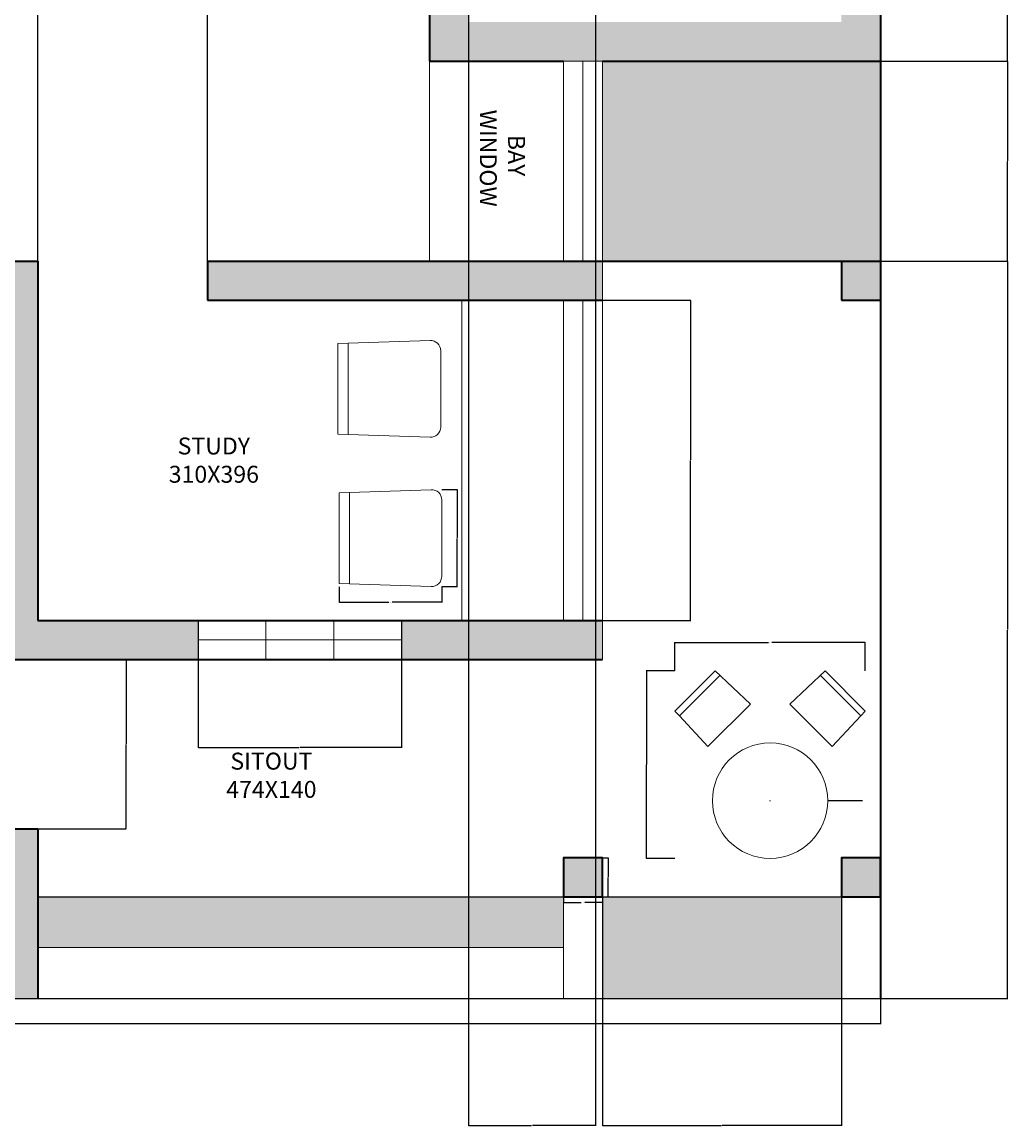
# Model space of a CAD drawing. Units: centimetres. Extents: x 2178 to 3635, y 1064 to 2635.
# Tile 4 of 9: x 3053 to 3635, y 1113 to 1765. Entities that reach past the tile are written whole.
import ezdxf

# ---------------------------------------------------------------- set-up
doc = ezdxf.new("R2010")
doc.units = ezdxf.units.CM
for name, color, linetype, lineweight in [('A-ANNO-DIMS', 2, 'Continuous', 18), ('A-ANNO-TEXT', 7, 'Continuous', 18), ('A-AREA-IDEN', 7, 'Continuous', 18), ('A-COLS', 7, 'Continuous', 35), ('A-FLOR', 7, 'Continuous', 25), ('A-FLOR-CASE', 32, 'Continuous', 18), ('A-FLOR-PATT', 95, 'Continuous', 13), ('A-FLOR-STRS', 7, 'Continuous', 18), ('A-FURN', 42, 'Continuous', 18), ('A-GLAZ', 4, 'Continuous', 18), ('A-WALL', 7, 'Continuous', 35)]:
    doc.layers.add(name, color=color, linetype=linetype, lineweight=lineweight)
doc.layers.add('A-WALL-PATT', color=18, linetype='Continuous', lineweight=13, true_color=0x000000)
doc.styles.get("Standard").update_dxf_attribs({"font": 'arial.ttf'})
doc.dimstyles.get("Standard").update_dxf_attribs({"dimtxt": 0.18, "dimasz": 0.18, "dimexe": 0.18, "dimexo": 0.0625, "dimgap": 0.09, "dimtad": 0, "dimtih": 1, "dimtoh": 1, "dimdec": 4, "dimzin": 0, "dimdsep": 46, "dimtxsty": 'Standard', "dimcen": 0.09, "dimadec": 0, "dimazin": 0, "dimtfac": 1, "dimtdec": 4, "dimtofl": 0, "dimtmove": 0, "dimatfit": 3, "dimfxl": 1, "dimtolj": 1, "dimtzin": 0, "dimarcsym": 0})

# ---------------------------------------------------------------- blocks, each defined once
blk = doc.blocks.new('chair')
for p, q in [((3410.95, 1354.53), (3434.84, 1378.41)), ((3434.84, 1378.41), (3410.95, 1354.53)), ((3494.17, 1378.41), (3518.06, 1354.53)), ((3518.06, 1354.53), (3494.17, 1378.41))]:
    blk.add_line(p, q)
for points in [[(3432.06, 1381.01), (3452.88, 1361.54), (3427.83, 1336.49), (3410.95, 1354.53), (3408.36, 1357.3)], [(3496.95, 1381.01), (3476.13, 1361.54), (3501.18, 1336.49), (3518.06, 1354.53), (3520.65, 1357.3)]]:
    blk.add_lwpolyline(points, close=True)
blk.add_circle((3464.51, 1304.51), 34.04)
blk = doc.blocks.new('c')
blk.add_lwpolyline([(3808.85, 1833.77), (3776.18, 1834.86), (3776.18, 1867.04), (3808.85, 1868.12, -0.424007), (3812.61, 1864.48), (3812.61, 1837.41, -0.424007)], format="xyb", close=True)
blk.add_lwpolyline([(3779.83, 1867.16), (3779.83, 1834.74)])
blk = doc.blocks.new('COL-0230-SQ')
blk.add_lwpolyline([(0, 0), (23, 0), (23, 23), (0, 23)], close=True)
blk = doc.blocks.new('*D20')
at = {"layer": 'A-ANNO-DIMS', "color": 0, "lineweight": -2, "transparency": 16777216}
for p, q in [((3240.31, 1431.49), (3240.31, 1422.28)), ((3300.89, 1431.49), (3300.89, 1422.28)), ((3240.49, 1422.46), (3269.64, 1422.46)), ((3300.71, 1422.46), (3271.55, 1422.46))]:
    blk.add_line(p, q, dxfattribs=at)
at = {"layer": 'A-ANNO-DIMS', "color": 0, "transparency": 16777216}
for points in [[(3240.49, 1422.49), (3240.49, 1422.43), (3240.31, 1422.46)], [(3300.71, 1422.49), (3300.71, 1422.43), (3300.89, 1422.46)]]:
    blk.add_solid(points, dxfattribs=at)
at = {"layer": 'Defpoints', "color": 0, "transparency": 16777216}
for p in [(3240.31, 1431.55), (3300.89, 1431.55), (3300.89, 1422.46)]:
    blk.add_point(p, dxfattribs=at)
at = {"layer": 'A-ANNO-DIMS', "color": 0, "transparency": 16777216, "insert": (3270.6, 1422.46), "char_height": 0.18, "attachment_point": 5}
blk.add_mtext('\\A1;CHAIR 61 TYP.', dxfattribs=at)
blk = doc.blocks.new('*D21')
at = {"layer": 'A-ANNO-DIMS', "color": 0, "lineweight": -2, "transparency": 16777216}
for p, q in [((3300.95, 1488.8), (3310.16, 1488.8)), ((3309.98, 1488.62), (3309.98, 1460.36)), ((3309.98, 1431.73), (3309.98, 1459.99)), ((3300.95, 1431.55), (3310.16, 1431.55))]:
    blk.add_line(p, q, dxfattribs=at)
at = {"layer": 'A-ANNO-DIMS', "color": 0, "transparency": 16777216}
for points in [[(3309.95, 1488.62), (3310.01, 1488.62), (3309.98, 1488.8)], [(3309.95, 1431.73), (3310.01, 1431.73), (3309.98, 1431.55)]]:
    blk.add_solid(points, dxfattribs=at)
at = {"layer": 'Defpoints', "color": 0, "transparency": 16777216}
for p in [(3300.89, 1488.8), (3309.98, 1488.8), (3300.89, 1431.55)]:
    blk.add_point(p, dxfattribs=at)
at = {"layer": 'A-ANNO-DIMS', "color": 0, "transparency": 16777216, "insert": (3309.98, 1460.17), "char_height": 0.18, "attachment_point": 5}
blk.add_mtext('\\A1;57 TYP.', dxfattribs=at)
blk = doc.blocks.new('*D38')
at = {"layer": 'A-ANNO-DIMS', "color": 0, "lineweight": -2, "transparency": 16777216}
for p, q in [((3372.6, 1248.53), (3372.6, 1244.96)), ((3372.78, 1245.14), (3383, 1245.14)), ((3395.42, 1245.14), (3385.21, 1245.14)), ((3395.6, 1248.53), (3395.6, 1244.96))]:
    blk.add_line(p, q, dxfattribs=at)
at = {"layer": 'A-ANNO-DIMS', "color": 0, "transparency": 16777216}
for points in [[(3372.78, 1245.17), (3372.78, 1245.11), (3372.6, 1245.14)], [(3395.42, 1245.17), (3395.42, 1245.11), (3395.6, 1245.14)]]:
    blk.add_solid(points, dxfattribs=at)
at = {"layer": 'Defpoints', "color": 0, "transparency": 16777216}
for p in [(3372.6, 1248.59), (3395.6, 1248.59), (3395.6, 1245.14)]:
    blk.add_point(p, dxfattribs=at)
at = {"layer": 'A-ANNO-DIMS', "color": 0, "transparency": 16777216, "insert": (3384.1, 1245.14), "char_height": 0.18, "attachment_point": 5}
blk.add_mtext('\\A1;COLUMN 23 TYP.', dxfattribs=at)
blk = doc.blocks.new('*D39')
at = {"layer": 'A-ANNO-DIMS', "color": 0, "lineweight": -2, "transparency": 16777216}
for p, q in [((3395.67, 1271.59), (3399.23, 1271.59)), ((3399.05, 1271.41), (3399.05, 1260.27)), ((3399.05, 1248.77), (3399.05, 1259.91)), ((3395.67, 1248.59), (3399.23, 1248.59))]:
    blk.add_line(p, q, dxfattribs=at)
at = {"layer": 'A-ANNO-DIMS', "color": 0, "transparency": 16777216}
for points in [[(3399.02, 1271.41), (3399.08, 1271.41), (3399.05, 1271.59)], [(3399.02, 1248.77), (3399.08, 1248.77), (3399.05, 1248.59)]]:
    blk.add_solid(points, dxfattribs=at)
at = {"layer": 'Defpoints', "color": 0, "transparency": 16777216}
for p in [(3395.6, 1271.59), (3399.05, 1271.59), (3395.6, 1248.59)]:
    blk.add_point(p, dxfattribs=at)
at = {"layer": 'A-ANNO-DIMS', "color": 0, "transparency": 16777216, "insert": (3399.05, 1260.09), "char_height": 0.18, "attachment_point": 5}
blk.add_mtext('\\A1;23 TYP.', dxfattribs=at)
blk = doc.blocks.new('*D42')
at = {"layer": 'A-ANNO-DIMS', "color": 0, "lineweight": -2, "transparency": 16777216}
for p, q in [((3438.42, 1381.84), (3438.42, 1398.8)), ((3438.6, 1398.62), (3493.59, 1398.62)), ((3550.53, 1398.62), (3495.54, 1398.62)), ((3550.71, 1381.84), (3550.71, 1398.8))]:
    blk.add_line(p, q, dxfattribs=at)
at = {"layer": 'A-ANNO-DIMS', "color": 0, "transparency": 16777216}
for points in [[(3438.6, 1398.65), (3438.6, 1398.59), (3438.42, 1398.62)], [(3550.53, 1398.65), (3550.53, 1398.59), (3550.71, 1398.62)]]:
    blk.add_solid(points, dxfattribs=at)
at = {"layer": 'Defpoints', "color": 0, "transparency": 16777216}
for p in [(3550.71, 1398.62), (3438.42, 1381.78), (3550.71, 1381.78)]:
    blk.add_point(p, dxfattribs=at)
at = {"layer": 'A-ANNO-DIMS', "color": 0, "transparency": 16777216, "insert": (3494.56, 1398.62), "char_height": 0.18, "attachment_point": 5}
blk.add_mtext('\\A1;PATIO SET 112', dxfattribs=at)
blk = doc.blocks.new('*D43')
at = {"layer": 'A-ANNO-DIMS', "color": 0, "lineweight": -2, "transparency": 16777216}
for p, q in [((3438.35, 1381.78), (3421.39, 1381.78)), ((3421.57, 1381.6), (3421.57, 1326.69)), ((3421.57, 1271.43), (3421.57, 1326.33)), ((3438.35, 1271.25), (3421.39, 1271.25))]:
    blk.add_line(p, q, dxfattribs=at)
at = {"layer": 'A-ANNO-DIMS', "color": 0, "transparency": 16777216}
for points in [[(3421.54, 1381.6), (3421.6, 1381.6), (3421.57, 1381.78)], [(3421.54, 1271.43), (3421.6, 1271.43), (3421.57, 1271.25)]]:
    blk.add_solid(points, dxfattribs=at)
at = {"layer": 'Defpoints', "color": 0, "transparency": 16777216}
for p in [(3421.57, 1381.78), (3438.42, 1381.78), (3438.42, 1271.25)]:
    blk.add_point(p, dxfattribs=at)
at = {"layer": 'A-ANNO-DIMS', "color": 0, "transparency": 16777216, "insert": (3421.57, 1326.51), "char_height": 0.18, "attachment_point": 5}
blk.add_mtext('\\A1;111', dxfattribs=at)
blk = doc.blocks.new('*D46')
at = {"layer": 'A-ANNO-DIMS', "color": 0, "lineweight": -2, "transparency": 16777216}
for p, q in [((2253.6, 1248.53), (2253.6, 1173.41)), ((3559.6, 1248.53), (3559.6, 1173.41)), ((2253.78, 1173.59), (2906.25, 1173.59)), ((3559.42, 1173.59), (2906.95, 1173.59))]:
    blk.add_line(p, q, dxfattribs=at)
at = {"layer": 'A-ANNO-DIMS', "color": 0, "transparency": 16777216}
for points in [[(2253.78, 1173.62), (2253.78, 1173.56), (2253.6, 1173.59)], [(3559.42, 1173.62), (3559.42, 1173.56), (3559.6, 1173.59)]]:
    blk.add_solid(points, dxfattribs=at)
at = {"layer": 'Defpoints', "color": 0, "transparency": 16777216}
for p in [(2253.6, 1248.59), (3559.6, 1248.59), (2253.6, 1173.59)]:
    blk.add_point(p, dxfattribs=at)
at = {"layer": 'A-ANNO-DIMS', "color": 0, "transparency": 16777216, "insert": (2906.6, 1173.59), "char_height": 0.18, "attachment_point": 5}
blk.add_mtext('\\A1;1306', dxfattribs=at)
blk = doc.blocks.new('*D58')
at = {"layer": 'A-ANNO-DIMS', "color": 0, "lineweight": -2, "transparency": 16777216}
for p, q in [((3559.67, 1797.09), (3634.78, 1797.09)), ((3634.6, 1796.91), (3634.6, 1769.52)), ((3634.6, 1741.77), (3634.6, 1769.16)), ((3559.67, 1741.59), (3634.78, 1741.59))]:
    blk.add_line(p, q, dxfattribs=at)
at = {"layer": 'A-ANNO-DIMS', "color": 0, "transparency": 16777216}
for points in [[(3634.57, 1796.91), (3634.63, 1796.91), (3634.6, 1797.09)], [(3634.57, 1741.77), (3634.63, 1741.77), (3634.6, 1741.59)]]:
    blk.add_solid(points, dxfattribs=at)
at = {"layer": 'Defpoints', "color": 0, "transparency": 16777216}
for p in [(3559.6, 1797.09), (3634.6, 1797.09), (3559.6, 1741.59)]:
    blk.add_point(p, dxfattribs=at)
at = {"layer": 'A-ANNO-DIMS', "color": 0, "transparency": 16777216, "insert": (3634.6, 1769.34), "char_height": 0.18, "attachment_point": 5}
blk.add_mtext('\\A1;55.5', dxfattribs=at)
blk = doc.blocks.new('*D59')
at = {"layer": 'A-ANNO-DIMS', "color": 0, "lineweight": -2, "transparency": 16777216}
for p, q in [((3559.67, 1741.59), (3634.78, 1741.59)), ((3634.6, 1741.41), (3634.6, 1682.77)), ((3634.6, 1623.77), (3634.6, 1682.41)), ((3559.67, 1623.59), (3634.78, 1623.59))]:
    blk.add_line(p, q, dxfattribs=at)
at = {"layer": 'A-ANNO-DIMS', "color": 0, "transparency": 16777216}
for points in [[(3634.57, 1741.41), (3634.63, 1741.41), (3634.6, 1741.59)], [(3634.57, 1623.77), (3634.63, 1623.77), (3634.6, 1623.59)]]:
    blk.add_solid(points, dxfattribs=at)
at = {"layer": 'Defpoints', "color": 0, "transparency": 16777216}
for p in [(3559.6, 1741.59), (3634.6, 1741.59), (3559.6, 1623.59)]:
    blk.add_point(p, dxfattribs=at)
at = {"layer": 'A-ANNO-DIMS', "color": 0, "transparency": 16777216, "insert": (3634.6, 1682.59), "char_height": 0.18, "attachment_point": 5}
blk.add_mtext('\\A1;118', dxfattribs=at)
blk = doc.blocks.new('*D60')
at = {"layer": 'A-ANNO-DIMS', "color": 0, "lineweight": -2, "transparency": 16777216}
for p, q in [((3559.67, 1623.59), (3634.78, 1623.59)), ((3634.6, 1623.41), (3634.6, 1406.27)), ((3634.6, 1188.77), (3634.6, 1405.91)), ((3559.67, 1188.59), (3634.78, 1188.59))]:
    blk.add_line(p, q, dxfattribs=at)
at = {"layer": 'A-ANNO-DIMS', "color": 0, "transparency": 16777216}
for points in [[(3634.57, 1623.41), (3634.63, 1623.41), (3634.6, 1623.59)], [(3634.57, 1188.77), (3634.63, 1188.77), (3634.6, 1188.59)]]:
    blk.add_solid(points, dxfattribs=at)
at = {"layer": 'Defpoints', "color": 0, "transparency": 16777216}
for p in [(3559.6, 1623.59), (3634.6, 1623.59), (3559.6, 1188.59)]:
    blk.add_point(p, dxfattribs=at)
at = {"layer": 'A-ANNO-DIMS', "color": 0, "transparency": 16777216, "insert": (3634.6, 1406.09), "char_height": 0.18, "attachment_point": 5}
blk.add_mtext('\\A1;435', dxfattribs=at)
blk = doc.blocks.new('*D62')
at = {"layer": 'A-ANNO-DIMS', "color": 0, "lineweight": -2, "transparency": 16777216}
for p, q in [((3062.6, 1623.65), (3062.6, 2634.77)), ((3062.78, 2634.59), (3112.32, 2634.59)), ((3162.42, 2634.59), (3112.88, 2634.59)), ((3162.6, 1623.65), (3162.6, 2634.77))]:
    blk.add_line(p, q, dxfattribs=at)
at = {"layer": 'A-ANNO-DIMS', "color": 0, "transparency": 16777216}
for points in [[(3062.78, 2634.62), (3062.78, 2634.56), (3062.6, 2634.59)], [(3162.42, 2634.62), (3162.42, 2634.56), (3162.6, 2634.59)]]:
    blk.add_solid(points, dxfattribs=at)
at = {"layer": 'Defpoints', "color": 0, "transparency": 16777216}
for p in [(3162.6, 2634.59), (3062.6, 1623.59), (3162.6, 1623.59)]:
    blk.add_point(p, dxfattribs=at)
at = {"layer": 'A-ANNO-DIMS', "color": 0, "transparency": 16777216, "insert": (3112.6, 2634.59), "char_height": 0.18, "attachment_point": 5}
blk.add_mtext('\\A1;100', dxfattribs=at)
blk = doc.blocks.new('*D67')
at = {"layer": 'A-ANNO-DIMS', "color": 0, "lineweight": -2, "transparency": 16777216}
for p, q in [((3316.6, 1927.53), (3316.6, 1113.41)), ((3391.6, 1927.53), (3391.6, 1113.41)), ((3316.78, 1113.59), (3353.89, 1113.59)), ((3391.42, 1113.59), (3354.32, 1113.59))]:
    blk.add_line(p, q, dxfattribs=at)
at = {"layer": 'A-ANNO-DIMS', "color": 0, "transparency": 16777216}
for points in [[(3316.78, 1113.62), (3316.78, 1113.56), (3316.6, 1113.59)], [(3391.42, 1113.62), (3391.42, 1113.56), (3391.6, 1113.59)]]:
    blk.add_solid(points, dxfattribs=at)
at = {"layer": 'Defpoints', "color": 0, "transparency": 16777216}
for p in [(3316.6, 1927.59), (3391.6, 1927.59), (3391.6, 1113.59)]:
    blk.add_point(p, dxfattribs=at)
at = {"layer": 'A-ANNO-DIMS', "color": 0, "transparency": 16777216, "insert": (3354.1, 1113.59), "char_height": 0.18, "attachment_point": 5}
blk.add_mtext('\\A1;75', dxfattribs=at)
blk = doc.blocks.new('*D68')
at = {"layer": 'A-ANNO-DIMS', "color": 0, "lineweight": -2, "transparency": 16777216}
for p, q in [((3372.67, 1600.59), (3447.78, 1600.59)), ((3447.6, 1600.41), (3447.6, 1506.27)), ((3447.6, 1411.77), (3447.6, 1505.91)), ((3372.67, 1411.59), (3447.78, 1411.59))]:
    blk.add_line(p, q, dxfattribs=at)
at = {"layer": 'A-ANNO-DIMS', "color": 0, "transparency": 16777216}
for points in [[(3447.57, 1600.41), (3447.63, 1600.41), (3447.6, 1600.59)], [(3447.57, 1411.77), (3447.63, 1411.77), (3447.6, 1411.59)]]:
    blk.add_solid(points, dxfattribs=at)
at = {"layer": 'Defpoints', "color": 0, "transparency": 16777216}
for p in [(3372.6, 1600.59), (3372.6, 1411.59), (3447.6, 1411.59)]:
    blk.add_point(p, dxfattribs=at)
at = {"layer": 'A-ANNO-DIMS', "color": 0, "transparency": 16777216, "insert": (3447.6, 1506.09), "char_height": 0.18, "attachment_point": 5}
blk.add_mtext('\\A1;189', dxfattribs=at)
blk = doc.blocks.new('*D78')
at = {"layer": 'A-ANNO-DIMS', "color": 0, "lineweight": -2, "transparency": 16777216}
for p, q in [((3039.67, 1388.59), (3114.78, 1388.59)), ((3114.6, 1388.41), (3114.6, 1338.77)), ((3114.6, 1288.77), (3114.6, 1338.41)), ((3039.67, 1288.59), (3114.78, 1288.59))]:
    blk.add_line(p, q, dxfattribs=at)
at = {"layer": 'A-ANNO-DIMS', "color": 0, "transparency": 16777216}
for points in [[(3114.57, 1388.41), (3114.63, 1388.41), (3114.6, 1388.59)], [(3114.57, 1288.77), (3114.63, 1288.77), (3114.6, 1288.59)]]:
    blk.add_solid(points, dxfattribs=at)
at = {"layer": 'Defpoints', "color": 0, "transparency": 16777216}
for p in [(3039.6, 1388.59), (3039.6, 1288.59), (3114.6, 1288.59)]:
    blk.add_point(p, dxfattribs=at)
at = {"layer": 'A-ANNO-DIMS', "color": 0, "transparency": 16777216, "insert": (3114.6, 1338.59), "char_height": 0.18, "attachment_point": 5}
blk.add_mtext('\\A1;100', dxfattribs=at)
blk = doc.blocks.new('*D79')
at = {"layer": 'A-ANNO-DIMS', "color": 0, "lineweight": -2, "transparency": 16777216}
for p, q in [((3395.6, 1248.53), (3395.6, 1113.41)), ((3536.6, 1248.53), (3536.6, 1113.41)), ((3395.78, 1113.59), (3465.84, 1113.59)), ((3536.42, 1113.59), (3466.37, 1113.59))]:
    blk.add_line(p, q, dxfattribs=at)
at = {"layer": 'A-ANNO-DIMS', "color": 0, "transparency": 16777216}
for points in [[(3395.78, 1113.62), (3395.78, 1113.56), (3395.6, 1113.59)], [(3536.42, 1113.62), (3536.42, 1113.56), (3536.6, 1113.59)]]:
    blk.add_solid(points, dxfattribs=at)
at = {"layer": 'Defpoints', "color": 0, "transparency": 16777216}
for p in [(3395.6, 1248.59), (3536.6, 1248.59), (3536.6, 1113.59)]:
    blk.add_point(p, dxfattribs=at)
at = {"layer": 'A-ANNO-DIMS', "color": 0, "transparency": 16777216, "insert": (3466.1, 1113.59), "char_height": 0.18, "attachment_point": 5}
blk.add_mtext('\\A1;141', dxfattribs=at)
blk = doc.blocks.new('*D80')
at = {"layer": 'A-ANNO-DIMS', "color": 0, "lineweight": -2, "transparency": 16777216}
for p, q in [((3157.1, 1411.53), (3157.1, 1336.41)), ((3277.1, 1411.53), (3277.1, 1336.41)), ((3157.28, 1336.59), (3216.82, 1336.59)), ((3276.92, 1336.59), (3217.38, 1336.59))]:
    blk.add_line(p, q, dxfattribs=at)
at = {"layer": 'A-ANNO-DIMS', "color": 0, "transparency": 16777216}
for points in [[(3157.28, 1336.62), (3157.28, 1336.56), (3157.1, 1336.59)], [(3276.92, 1336.62), (3276.92, 1336.56), (3277.1, 1336.59)]]:
    blk.add_solid(points, dxfattribs=at)
at = {"layer": 'Defpoints', "color": 0, "transparency": 16777216}
for p in [(3157.1, 1411.59), (3277.1, 1411.59), (3157.1, 1336.59)]:
    blk.add_point(p, dxfattribs=at)
at = {"layer": 'A-ANNO-DIMS', "color": 0, "transparency": 16777216, "insert": (3217.1, 1336.59), "char_height": 0.18, "attachment_point": 5}
blk.add_mtext('\\A1;120', dxfattribs=at)
blk = doc.blocks.new('*D85')
at = {"layer": 'A-ANNO-DIMS', "color": 0, "lineweight": -2, "transparency": 16777216}
for p, q in [((3494.47, 1305.28), (3494.65, 1305.28)), ((3494.56, 1305.19), (3494.56, 1305.37)), ((3549.02, 1305.28), (3528.78, 1305.28))]:
    blk.add_line(p, q, dxfattribs=at)
at = {"layer": 'A-ANNO-DIMS', "color": 0, "transparency": 16777216}
blk.add_solid([(3528.78, 1305.31), (3528.78, 1305.25), (3528.6, 1305.28)], dxfattribs=at)
at = {"layer": 'Defpoints', "color": 0, "transparency": 16777216}
for p in [(3460.53, 1305.28), (3528.6, 1305.28)]:
    blk.add_point(p, dxfattribs=at)
at = {"layer": 'A-ANNO-DIMS', "color": 0, "transparency": 16777216, "insert": (3549.51, 1305.28), "char_height": 0.18, "attachment_point": 5}
blk.add_mtext('\\A1;∅68.07', dxfattribs=at)

msp = doc.modelspace()

# ---------------------------------------------------------------- hatches: boundary and pattern name
at = {"layer": 'A-FLOR-PATT'}
h = msp.add_hatch(color=256, dxfattribs=at)
h.dxf.hatch_style = 1
h.paths.add_polyline_path([(3559.605, 1741.59), (3395.605, 1741.59), (3395.605, 1623.59), (3559.605, 1623.59)])
h.paths.add_polyline_path([(3536.605, 1248.59), (3395.605, 1248.59), (3395.605, 1188.59), (3536.605, 1188.59)])
h.paths.add_polyline_path([(2636.605, 1248.59), (2253.605, 1248.59), (2253.605, 1188.59), (2636.605, 1188.59)])
at = {"layer": 'A-WALL-PATT'}
h = msp.add_hatch(color=256, dxfattribs=at)
h.dxf.hatch_style = 1
h.paths.add_polyline_path([(2276.605, 2499.59), (2253.605, 2499.59), (2253.605, 2476.59), (2276.605, 2476.59)])
h.paths.add_polyline_path([(2411.605, 2350.59), (2253.605, 2350.59), (2253.605, 2327.59), (2411.605, 2327.59)])
h.paths.add_polyline_path([(2276.605, 2252.59), (2253.605, 2252.59), (2253.605, 2020.59), (2276.605, 2020.59), (2276.605, 2093.59), (2561.605, 2093.59), (2561.605, 2116.59), (2276.605, 2116.59)])
h.paths.add_polyline_path([(2659.605, 1787.59), (2610.616, 1787.59), (2276.605, 1787.59), (2276.605, 1860.59), (2253.605, 1860.59), (2253.605, 1732.09), (2276.605, 1732.09), (2276.605, 1764.59), (2516.605, 1764.59), (2516.605, 1699.59), (2539.605, 1699.59), (2539.605, 1764.59), (2659.605, 1764.59)])
h.paths.add_polyline_path([(2539.605, 1624.59), (2276.605, 1624.59), (2276.605, 1657.09), (2253.605, 1657.09), (2253.605, 1561.59), (2276.605, 1561.59), (2276.605, 1601.59), (2539.605, 1601.59)])
h.paths.add_polyline_path([(2276.605, 1501.59), (2253.605, 1501.59), (2253.605, 1371.59), (2276.605, 1371.59)])
h.paths.add_polyline_path([(2376.605, 1271.59), (2276.605, 1271.59), (2276.605, 1311.59), (2253.605, 1311.59), (2253.605, 1248.59), (2376.605, 1248.59)])
h.paths.add_polyline_path([(2636.605, 1271.59), (2536.605, 1271.59), (2536.605, 1248.59), (2636.605, 1248.59)])
h.paths.add_polyline_path([(2659.605, 1600.59), (2919.605, 1600.59), (2919.605, 1623.59), (2636.605, 1623.59), (2636.605, 1188.59), (2659.605, 1188.59)])
h.paths.add_polyline_path([(2939.605, 1211.59), (2759.605, 1211.59), (2759.605, 1188.59), (2939.605, 1188.59)])
h.paths.add_polyline_path([(3062.605, 1288.59), (3039.605, 1288.59), (3039.605, 1188.59), (3062.605, 1188.59)])
h.paths.add_polyline_path([(3372.605, 1248.59), (3062.605, 1248.59), (3062.605, 1218.59), (3372.605, 1218.59)])
h.paths.add_polyline_path([(3395.605, 1271.59), (3372.605, 1271.59), (3372.605, 1248.59), (3395.605, 1248.59)])
h.paths.add_polyline_path([(3559.605, 1271.59), (3536.605, 1271.59), (3536.605, 1248.59), (3559.605, 1248.59)])
h.paths.add_polyline_path([(3559.605, 1623.59), (3536.605, 1623.59), (3536.605, 1600.59), (3559.605, 1600.59)])
h.paths.add_polyline_path([(3395.605, 1623.59), (3162.605, 1623.59), (3162.605, 1600.59), (3395.605, 1600.59)])
h.paths.add_polyline_path([(3395.605, 1411.59), (3277.1, 1411.59), (3277.1, 1388.59), (3395.605, 1388.59)])
h.paths.add_polyline_path([(3157.1, 1411.59), (3062.605, 1411.59), (3062.605, 1623.59), (3039.605, 1623.59), (3039.605, 1388.59), (3157.1, 1388.59)])
h.paths.add_polyline_path([(3559.605, 1797.09), (3536.605, 1797.09), (3536.605, 1764.59), (3316.605, 1764.59), (3316.605, 1927.59), (3293.605, 1927.59), (3293.605, 1741.59), (3372.605, 1741.59), (3395.605, 1741.59), (3559.605, 1741.59)])
h.paths.add_polyline_path([(3559.605, 1990.59), (3536.605, 1990.59), (3536.605, 1974.446), (3536.605, 1927.59), (3391.605, 1927.59), (3391.605, 1904.59), (3536.605, 1904.59), (3536.605, 1872.09), (3559.605, 1872.09)])
h.paths.add_polyline_path([(3559.605, 2180.59), (3536.605, 2180.59), (3536.605, 2050.59), (3559.605, 2050.59)])
h.paths.add_polyline_path([(3559.605, 2326.59), (3446.105, 2326.59), (3446.105, 2303.59), (3536.605, 2303.59), (3536.605, 2240.59), (3559.605, 2240.59)])
h.paths.add_polyline_path([(3286.105, 2326.59), (3195.605, 2326.59), (3195.605, 2499.59), (3082.605, 2499.59), (3082.605, 2476.59), (3172.605, 2476.59), (3172.605, 2116.59), (2809.605, 2116.59), (2809.605, 2093.59), (3172.605, 2093.59), (3172.605, 1904.59), (3195.605, 1904.59), (3195.605, 2303.59), (3286.105, 2303.59)])
h.paths.add_polyline_path([(2832.605, 2236.59), (2659.605, 2236.59), (2659.605, 2476.59), (2697.105, 2476.59), (2697.105, 2499.59), (2636.605, 2499.59), (2636.605, 2093.59), (2699.605, 2093.59), (2699.605, 2116.59), (2659.605, 2116.59), (2659.605, 2213.59), (2832.605, 2213.59)])
h.paths.add_polyline_path([(2832.605, 2476.59), (2922.605, 2476.59), (2922.605, 2499.59), (2772.105, 2499.59), (2772.105, 2476.59), (2809.605, 2476.59), (2809.605, 2311.59), (2832.605, 2311.59)])

# ---------------------------------------------------------------- linework, layer by layer
at = {"layer": 'A-COLS'}
for p, q in [((3536.605, 1623.59), (3536.605, 1600.59)), ((3536.605, 1600.59), (3559.605, 1600.59))]:
    msp.add_line(p, q, dxfattribs=at)
at = {"layer": 'A-FLOR'}
for p, q in [((3062.605, 1248.59), (3559.605, 1248.59)), ((2253.605, 1188.59), (3559.605, 1188.59))]:
    msp.add_line(p, q, dxfattribs=at)
at = {"layer": 'A-FLOR-CASE'}
for p, q in [((3293.605, 1741.59), (3293.605, 1623.59)), ((3312.605, 1600.59), (3312.605, 1411.59))]:
    msp.add_line(p, q, dxfattribs=at)
at = {"layer": 'A-FLOR-STRS'}
for p, q in [((3372.605, 1271.59), (3372.605, 1188.59)), ((3395.605, 1271.59), (3395.605, 1188.59)), ((3536.605, 1271.59), (3536.605, 1188.59)), ((3062.605, 1218.59), (3372.605, 1218.59))]:
    msp.add_line(p, q, dxfattribs=at)
at = {"layer": 'A-GLAZ'}
for p, q in [((3372.605, 1741.59), (3372.605, 1623.59)), ((3372.605, 1741.59), (3395.605, 1741.59)), ((3384.105, 1741.59), (3384.105, 1623.59)), ((3395.605, 1741.59), (3395.605, 1388.59)), ((3372.605, 1600.59), (3372.605, 1411.59)), ((3384.105, 1600.59), (3384.105, 1411.59)), ((3157.1, 1388.59), (3157.1, 1411.59)), ((3197.1, 1388.59), (3197.1, 1411.59)), ((3237.1, 1388.59), (3237.1, 1411.59)), ((3277.1, 1388.59), (3277.1, 1411.59)), ((3157.1, 1400.09), (3277.1, 1400.09))]:
    msp.add_line(p, q, dxfattribs=at)
at = {"layer": 'A-WALL'}
for p, q in [((3559.605, 2326.59), (3559.605, 1188.59)), ((3293.605, 1927.59), (3293.605, 1741.59)), ((3293.605, 1741.59), (3372.605, 1741.59)), ((3395.605, 1741.59), (3559.605, 1741.59)), ((3039.605, 1623.59), (3062.605, 1623.59)), ((3062.605, 1623.59), (3062.605, 1411.59)), ((3162.605, 1623.59), (3162.605, 1600.59)), ((3162.605, 1623.59), (3559.605, 1623.59)), ((3162.605, 1600.59), (3395.605, 1600.59)), ((3062.605, 1411.59), (3395.605, 1411.59)), ((3039.605, 1388.59), (3395.605, 1388.59)), ((3039.605, 1288.59), (3062.605, 1288.59)), ((3062.605, 1288.59), (3062.605, 1188.59))]:
    msp.add_line(p, q, dxfattribs=at)

# ---------------------------------------------------------------- block references
at = {"layer": 'A-COLS'}
for p in [(3372.605, 1248.59), (3536.605, 1248.59)]:
    msp.add_blockref('COL-0230-SQ', p, dxfattribs=at)
at = {"layer": 'A-FURN', "xscale": 1.663033133753634, "yscale": 1.663033133753634, "zscale": 1.663033133753634}
for p in [(-3040.281, -1529.969), (-3039.613, -1618.011)]:
    msp.add_blockref('c', p, dxfattribs=at)
at = {"layer": 'A-FURN'}
msp.add_blockref('chair', (30.059, 0.77), dxfattribs=at)

# ---------------------------------------------------------------- texts
at = {"layer": 'A-ANNO-TEXT', "insert": (3350, 1741.59), "char_height": 10, "attachment_point": 1, "rotation": 270}
msp.add_mtext_dynamic_manual_height_columns('\\pxqc;BAY\\P WINDOW', width=111.5542, gutter_width=12.5, heights=[0], dxfattribs=at)
at = {"layer": 'A-AREA-IDEN', "char_height": 10, "attachment_point": 1}
for s, insert in [('\\pxqc;STUDY\\P310X396', (3110.634, 1519.507)), ('\\pxqc;SITOUT\\P474X140', (3144.592, 1333.604))]:
    msp.add_mtext_dynamic_manual_height_columns(s, width=111.5542, gutter_width=12.5, heights=[0], dxfattribs=dict(at, insert=insert))

# ---------------------------------------------------------------- dimensions: what is measured, and where the dimension line sits
at = {"layer": 'A-ANNO-DIMS'}
for base, p1, p2, picture, middle in [((3162.605, 2634.59), (3062.605, 1623.59), (3162.605, 1623.59), '*D62', (3112.605, 2634.59)), ((3391.605, 1113.59), (3316.605, 1927.59), (3391.605, 1927.59), '*D67', (3354.105, 1113.59)), ((3536.605, 1113.59), (3395.605, 1248.59), (3536.605, 1248.59), '*D79', (3466.105, 1113.59))]:
    dim = msp.add_linear_dim(base=base, p1=p1, p2=p2, dimstyle='Standard', override={"dimdec": 0, "dimlfac": 1, "dimrnd": 0, "dimzin": 0, "dimdsep": 46, "dimlunit": 2}, dxfattribs=at)
    dim.commit()
    dim.dimension.update_dxf_attribs({"geometry": picture, "text_midpoint": middle})
for base, p1, p2, angle, override, picture, middle in [((3634.605, 1797.09), (3559.605, 1741.59), (3559.605, 1797.09), 90, {"dimdec": 1, "dimlfac": 1, "dimrnd": 0, "dimzin": 0, "dimdsep": 46, "dimlunit": 2}, '*D58', (3634.605, 1769.34)), ((3634.605, 1741.59), (3559.605, 1623.59), (3559.605, 1741.59), 90, {"dimdec": 0, "dimlfac": 1, "dimrnd": 0, "dimzin": 0, "dimdsep": 46, "dimlunit": 2}, '*D59', (3634.605, 1682.59)), ((3634.605, 1623.59), (3559.605, 1188.59), (3559.605, 1623.59), 90, {"dimdec": 0, "dimlfac": 1, "dimrnd": 0, "dimzin": 0, "dimdsep": 46, "dimlunit": 2}, '*D60', (3634.605, 1406.09)), ((3447.605, 1411.59), (3372.605, 1600.59), (3372.605, 1411.59), 270, {"dimdec": 0, "dimlfac": 1, "dimrnd": 0, "dimzin": 0, "dimdsep": 46, "dimlunit": 2}, '*D68', (3447.605, 1506.09)), ((3157.1, 1336.59), (3277.1, 1411.59), (3157.1, 1411.59), 180, {"dimdec": 0, "dimlfac": 1, "dimrnd": 0, "dimzin": 0, "dimdsep": 46, "dimlunit": 2}, '*D80', (3217.1, 1336.59)), ((3114.605, 1288.59), (3039.605, 1388.59), (3039.605, 1288.59), 270, {"dimdec": 0, "dimlfac": 1, "dimrnd": 0, "dimzin": 0, "dimdsep": 46, "dimlunit": 2}, '*D78', (3114.605, 1338.59)), ((3421.573, 1381.775), (3438.417, 1271.246), (3438.417, 1381.775), 90, {"dimdec": 0, "dimlfac": 1, "dimrnd": 0, "dimzin": 0, "dimdsep": 46, "dimlunit": 2}, '*D43', (3421.573, 1326.511)), ((2253.605, 1173.59), (3559.605, 1248.59), (2253.605, 1248.59), 180, {"dimdec": 0, "dimlfac": 1, "dimrnd": 0, "dimzin": 0, "dimdsep": 46, "dimlunit": 2}, '*D46', (2906.605, 1173.59))]:
    dim = msp.add_linear_dim(base=base, p1=p1, p2=p2, angle=angle, dimstyle='Standard', override=override, dxfattribs=at)
    dim.commit()
    dim.dimension.update_dxf_attribs({"geometry": picture, "text_midpoint": middle})
for base, p1, p2, picture, middle in [((3309.976, 1488.796), (3300.888, 1431.552), (3300.888, 1488.796), '*D21', (3309.976, 1460.174)), ((3399.055, 1271.59), (3395.605, 1248.59), (3395.605, 1271.59), '*D39', (3399.055, 1260.09))]:
    dim = msp.add_linear_dim(base=base, p1=p1, p2=p2, angle=90, text='<> TYP.', dimstyle='Standard', override={"dimdec": 0, "dimlfac": 1, "dimrnd": 0, "dimzin": 0, "dimdsep": 46, "dimlunit": 2}, dxfattribs=at)
    dim.commit()
    dim.dimension.update_dxf_attribs({"geometry": picture, "text_midpoint": middle})
for base, p1, p2, text, picture, middle in [((3300.888, 1422.465), (3240.307, 1431.552), (3300.888, 1431.552), 'CHAIR <> TYP.', '*D20', (3270.598, 1422.465)), ((3550.711, 1398.619), (3438.417, 1381.775), (3550.711, 1381.775), 'PATIO SET <>', '*D42', (3494.564, 1398.619)), ((3395.605, 1245.14), (3372.605, 1248.59), (3395.605, 1248.59), 'COLUMN <> TYP.', '*D38', (3384.105, 1245.14))]:
    dim = msp.add_linear_dim(base=base, p1=p1, p2=p2, text=text, dimstyle='Standard', override={"dimdec": 0, "dimlfac": 1, "dimrnd": 0, "dimzin": 0, "dimdsep": 46, "dimlunit": 2}, dxfattribs=at)
    dim.commit()
    dim.dimension.update_dxf_attribs({"geometry": picture, "text_midpoint": middle})
dim = msp.add_diameter_dim_2p(p1=(3460.529, 1305.281), p2=(3528.599, 1305.281), dimstyle='Standard', override={"dimdec": 2, "dimlfac": 1, "dimrnd": 0, "dimzin": 0, "dimdsep": 46, "dimlunit": 2}, dxfattribs=at)
dim.commit()
dim.dimension.update_dxf_attribs({"geometry": '*D85', "text_midpoint": (3549.021, 1305.281), "dimtype": 163})

doc.saveas('drawing.dxf')
